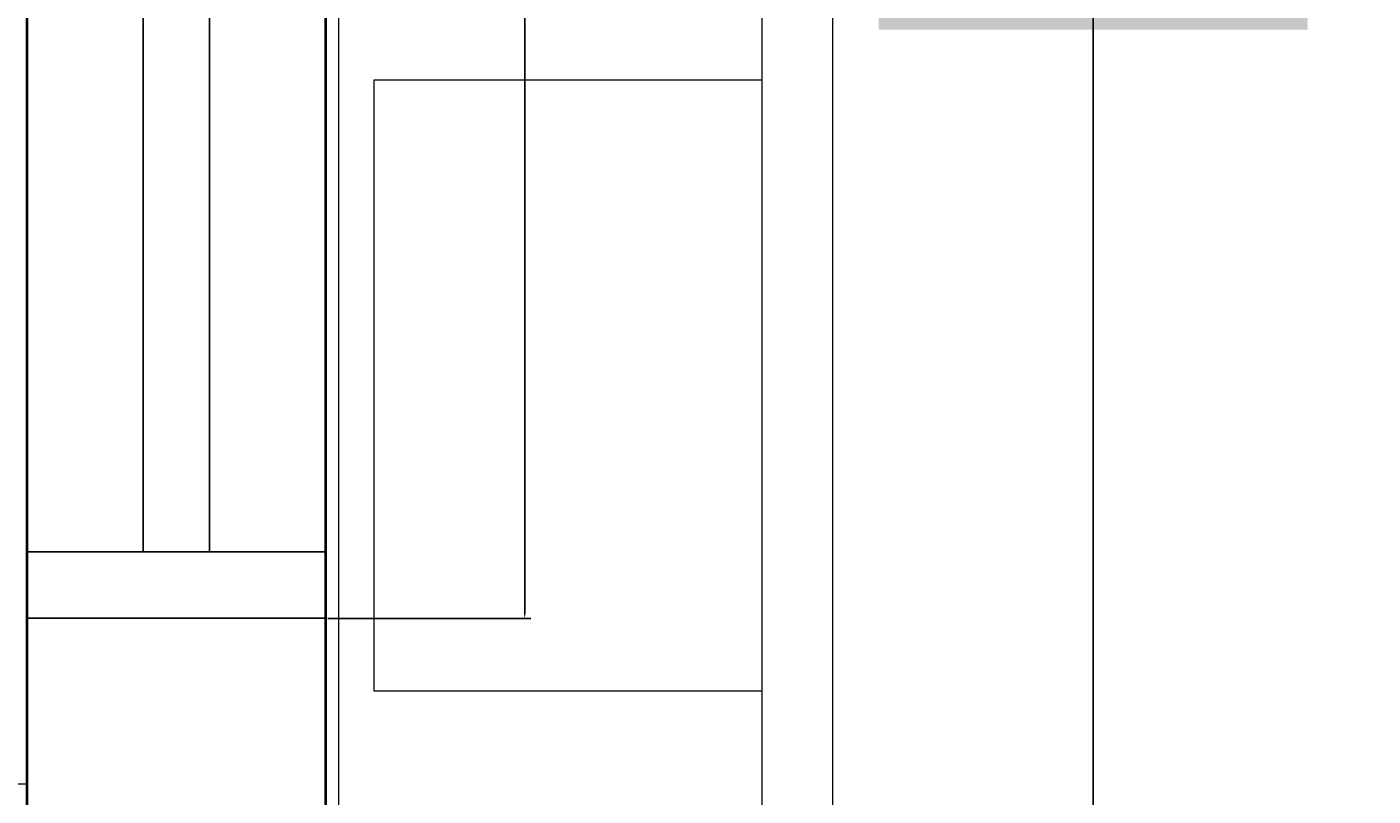
# Model space of a CAD drawing. Units: inches. Extents: x -301 to 715, y -607 to 364.
# Tile 71 of 141: x -205 to -164, y -26 to -3. Entities that reach past the tile are written whole.
import ezdxf

# ---------------------------------------------------------------- set-up
doc = ezdxf.new("R2010")
doc.units = ezdxf.units.IN
doc.header["$MEASUREMENT"] = 0
doc.linetypes.add('ACAD_ISO02W100', pattern=[15, 12, -3])
for name, color, linetype, lineweight in [('A-ANNO-DIMS', 2, 'Continuous', 18), ('A-FURN', 8, 'Continuous', 18), ('A-GLAZ', 2, 'Continuous', 25), ('A-GLAZ-OVHD', 2, 'ACAD_ISO02W100', 18), ('A-WALL', 3, 'Continuous', 40)]:
    doc.layers.add(name, color=color, linetype=linetype, lineweight=lineweight)
doc.styles.get("Standard").update_dxf_attribs({"font": 'arial.ttf'})
doc.dimstyles.get("Standard").update_dxf_attribs({"dimtxt": 0.18, "dimasz": 0.18, "dimexe": 0.18, "dimexo": 0.0625, "dimgap": 0.09, "dimtad": 0, "dimtih": 1, "dimtoh": 1, "dimdec": 1, "dimzin": 0, "dimdsep": 46, "dimlunit": 4, "dimtxsty": 'Standard', "dimcen": 0.09, "dimclrd": 3, "dimclre": 4, "dimclrt": 6, "dimadec": 0, "dimazin": 0, "dimtfac": 1, "dimtdec": 1, "dimtofl": 0, "dimtmove": 0, "dimatfit": 3, "dimfxl": 1, "dimtfill": 2, "dimtfillclr": 51, "dimtolj": 1, "dimtzin": 0, "dimarcsym": 0})

# ---------------------------------------------------------------- blocks, each defined once
blk = doc.blocks.new('Bed - Queen')
for p, q in [((0, 0), (59.99999, 0)), ((7.99999, -1.2), (28.79998, -1.2)), ((7.99999, -14.4), (7.99999, -1.2)), ((28.79998, -1.2), (28.79998, -14.4)), ((0, -14.4), (44.8, -14.4)), ((44.8, -16.8), (0, -16.8))]:
    blk.add_line(p, q)
blk = doc.blocks.new('*D56')
at = {"layer": 'A-ANNO-DIMS', "color": 0, "lineweight": -2, "transparency": 16777216}
for p, q in [((-195.541, 65.682), (-172.295, 65.682)), ((-172.475, 60.682), (-172.475, 0.778)), ((-172.475, -62.318), (-172.475, -2.414)), ((-195.541, -67.318), (-172.295, -67.318))]:
    blk.add_line(p, q, dxfattribs=at)
at = {"layer": 'A-ANNO-DIMS', "color": 0, "transparency": 16777216}
for points in [[(-173.308, 60.682), (-171.641, 60.682), (-172.475, 65.682)], [(-173.308, -62.318), (-171.641, -62.318), (-172.475, -67.318)]]:
    blk.add_solid(points, dxfattribs=at)
at = {"layer": 'Defpoints', "color": 0, "transparency": 16777216}
for p in [(-195.603, 65.682), (-172.475, 65.682), (-195.603, -67.318)]:
    blk.add_point(p, dxfattribs=at)
at = {"layer": 'A-ANNO-DIMS', "color": 0, "transparency": 16777216, "insert": (-172.475, -0.818), "char_height": 3, "attachment_point": 5, "bg_fill": 1, "box_fill_scale": 1.25, "bg_fill_color": 51, "bg_fill_transparency": 0}
blk.add_mtext('\\A1;11\'-1"', dxfattribs=at)
blk = doc.blocks.new('WIN-36-PLAN')
for p, q in [((0, 0), (0, 9)), ((2, 0), (2, 9)), ((20, 0), (20, 9)), ((38, 0), (38, 9)), ((40, 0), (40, 9)), ((2, 5.5), (38, 5.5)), ((2, 3.5), (38, 3.5))]:
    blk.add_line(p, q)
blk = doc.blocks.new('WIN-SHADE-50')
at = {"ltscale": 1.5}
for p, q in [((0, 0), (0, 12)), ((50, 12), (0, 12)), ((50, 0), (50, 12)), ((5, 0), (0, 0)), ((45, 0), (50, 0))]:
    blk.add_line(p, q, dxfattribs=at)
blk = doc.blocks.new('*D96')
at = {"layer": 'A-ANNO-DIMS', "color": 4, "lineweight": -2, "transparency": 16777216}
for p, q in [((-195.541, 19.182), (-189.423, 19.182)), ((-195.541, -20.818), (-189.423, -20.818))]:
    blk.add_line(p, q, dxfattribs=at)
at = {"layer": 'A-ANNO-DIMS', "color": 3, "lineweight": -2, "transparency": 16777216}
for p, q in [((-189.603, 19.002), (-189.603, -0.634)), ((-189.603, -20.638), (-189.603, -1.001))]:
    blk.add_line(p, q, dxfattribs=at)
at = {"layer": 'A-ANNO-DIMS', "color": 3, "transparency": 16777216}
for points in [[(-189.633, 19.002), (-189.573, 19.002), (-189.603, 19.182)], [(-189.633, -20.638), (-189.573, -20.638), (-189.603, -20.818)]]:
    blk.add_solid(points, dxfattribs=at)
at = {"layer": 'Defpoints', "color": 0, "transparency": 16777216}
for p in [(-195.603, 19.182), (-189.603, 19.182), (-195.603, -20.818)]:
    blk.add_point(p, dxfattribs=at)
at = {"layer": 'A-ANNO-DIMS', "color": 6, "transparency": 16777216, "insert": (-189.603, -0.818), "char_height": 0.18, "attachment_point": 5, "bg_fill": 1, "box_fill_scale": 1.25, "bg_fill_color": 51, "bg_fill_transparency": 0}
blk.add_mtext('\\A1;WINDOW 3\'-4" TYP.', dxfattribs=at)
blk = doc.blocks.new('*D151')
at = {"layer": 'A-ANNO-DIMS', "color": 4, "lineweight": -2, "transparency": 16777216}
for p, q in [((-204.603, -223.755), (-204.603, 359.612)), ((-45.603, -214.755), (-45.603, 359.612))]:
    blk.add_line(p, q, dxfattribs=at)
at = {"layer": 'A-ANNO-DIMS', "color": 3, "lineweight": -2, "transparency": 16777216}
for p, q in [((-204.423, 359.432), (-125.494, 359.432)), ((-45.783, 359.432), (-124.713, 359.432))]:
    blk.add_line(p, q, dxfattribs=at)
at = {"layer": 'A-ANNO-DIMS', "color": 3, "transparency": 16777216}
for points in [[(-204.423, 359.462), (-204.423, 359.402), (-204.603, 359.432)], [(-45.783, 359.462), (-45.783, 359.402), (-45.603, 359.432)]]:
    blk.add_solid(points, dxfattribs=at)
at = {"layer": 'Defpoints', "color": 0, "transparency": 16777216}
for p in [(-45.603, 359.432), (-45.603, -214.818), (-204.603, -223.818)]:
    blk.add_point(p, dxfattribs=at)
at = {"layer": 'A-ANNO-DIMS', "color": 6, "transparency": 16777216, "insert": (-125.103, 359.432), "char_height": 0.18, "attachment_point": 5, "bg_fill": 1, "box_fill_scale": 1.25, "bg_fill_color": 51, "bg_fill_transparency": 0}
blk.add_mtext('\\A1;13\'-3"', dxfattribs=at)

msp = doc.modelspace()

# ---------------------------------------------------------------- linework, layer by layer
at = {"layer": 'A-WALL'}
for p, q in [((-204.603, 71.682), (-204.603, -67.318)), ((-195.603, 65.682), (-195.603, -67.318))]:
    msp.add_line(p, q, dxfattribs=at)

# ---------------------------------------------------------------- block references
at = {"layer": 'A-FURN', "xscale": 0.8856750462000775, "yscale": 0.8856750462000775, "zscale": 0.8856750462000775, "rotation": 90}
msp.add_blockref('Bed - Queen', (-195.207, -30.095), dxfattribs=at)
at = {"layer": 'A-GLAZ', "rotation": 90.00000000000043}
msp.add_blockref('WIN-36-PLAN', (-195.603, -20.817), dxfattribs=at)
at = {"layer": 'A-GLAZ-OVHD', "rotation": 90.00000000000011}
msp.add_blockref('WIN-SHADE-50', (-204.603, -25.817), dxfattribs=at)

# ---------------------------------------------------------------- dimensions: what is measured, and where the dimension line sits
at = {"layer": 'A-ANNO-DIMS'}
dim = msp.add_linear_dim(base=(-45.603, 359.432), p1=(-204.603, -223.818), p2=(-45.603, -214.818), dimstyle='Standard', override={"dimdec": 1, "dimlfac": 1, "dimrnd": 0, "dimzin": 1, "dimdsep": 46, "dimlunit": 4, "dimfrac": 2}, dxfattribs=at)
dim.commit()
dim.dimension.update_dxf_attribs({"geometry": '*D151', "text_midpoint": (-125.103, 359.432)})
dim = msp.add_linear_dim(base=(-172.475, 65.682), p1=(-195.603, -67.318), p2=(-195.603, 65.682), angle=90, dimstyle='Standard', override={"dimtxt": 3, "dimasz": 5, "dimclrd": 0, "dimclre": 0, "dimclrt": 0}, dxfattribs=at)
dim.commit()
dim.dimension.update_dxf_attribs({"geometry": '*D56', "text_midpoint": (-172.475, -0.818)})
dim = msp.add_linear_dim(base=(-189.603, 19.182), p1=(-195.603, -20.818), p2=(-195.603, 19.182), angle=90, text='WINDOW <> TYP.', dimstyle='Standard', override={"dimdec": 1, "dimlfac": 1, "dimrnd": 0, "dimzin": 1, "dimdsep": 46, "dimlunit": 4, "dimfrac": 2}, dxfattribs=at)
dim.commit()
dim.dimension.update_dxf_attribs({"geometry": '*D96', "text_midpoint": (-189.603, -0.818)})

doc.saveas('drawing.dxf')
